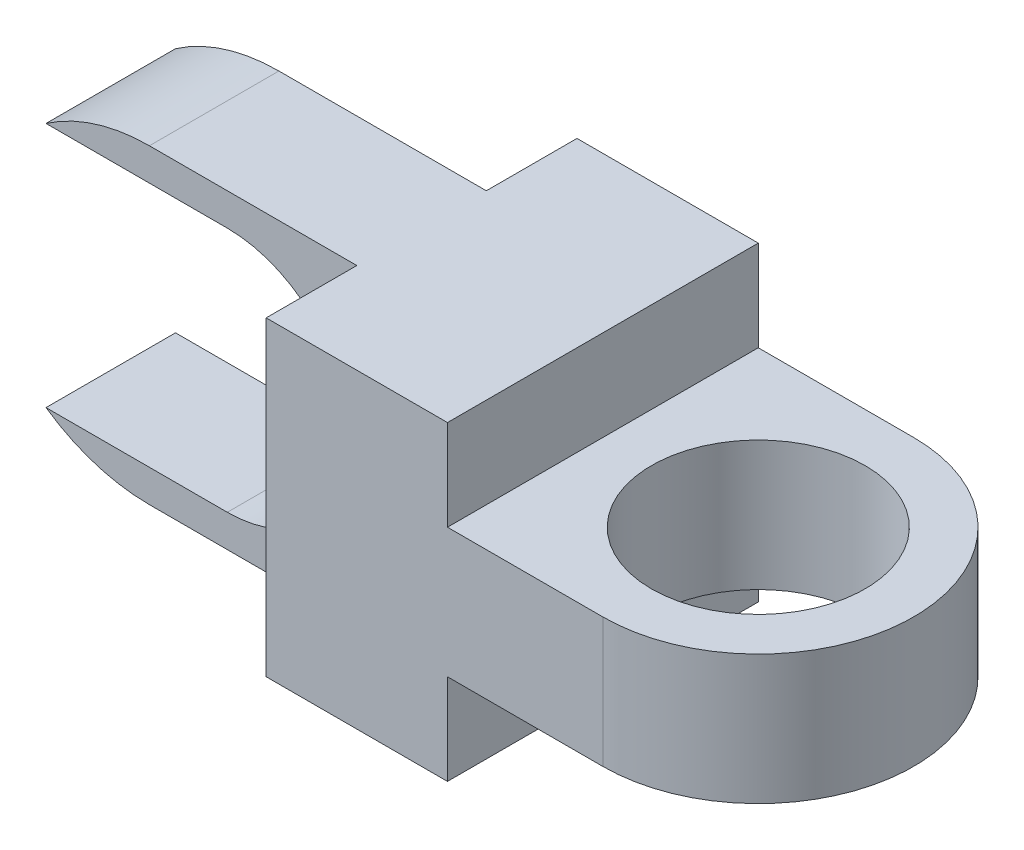
ISO-10303-21;
HEADER;
FILE_DESCRIPTION(('STEP AP214'),'2;1');
FILE_NAME('part.step','',(''),(''),'','','');
FILE_SCHEMA(('AUTOMOTIVE_DESIGN { 1 0 10303 214 1 1 1 1 }'));
ENDSEC;
DATA;
#1=APPLICATION_CONTEXT('core data for automotive mechanical design processes');
#2=APPLICATION_PROTOCOL_DEFINITION('international standard','automotive_design',2000,#1);
#3=PRODUCT_CONTEXT('',#1,'mechanical');
#4=PRODUCT('Part','Part','',(#3));
#5=PRODUCT_RELATED_PRODUCT_CATEGORY('part','',(#4));
#6=PRODUCT_DEFINITION_FORMATION('','',#4);
#7=PRODUCT_DEFINITION_CONTEXT('part definition',#1,'design');
#8=PRODUCT_DEFINITION('design','',#6,#7);
#9=PRODUCT_DEFINITION_SHAPE('','',#8);
#10=(LENGTH_UNIT() NAMED_UNIT(*) SI_UNIT(.MILLI.,.METRE.));
#11=(NAMED_UNIT(*) PLANE_ANGLE_UNIT() SI_UNIT($,.RADIAN.));
#12=(NAMED_UNIT(*) SI_UNIT($,.STERADIAN.) SOLID_ANGLE_UNIT());
#13=UNCERTAINTY_MEASURE_WITH_UNIT(LENGTH_MEASURE(1.E-05),#10,'distance_accuracy_value','');
#14=(GEOMETRIC_REPRESENTATION_CONTEXT(3) GLOBAL_UNCERTAINTY_ASSIGNED_CONTEXT((#13)) GLOBAL_UNIT_ASSIGNED_CONTEXT((#10,
#11,#12)) REPRESENTATION_CONTEXT('',''));
#15=CARTESIAN_POINT('',(0.,0.,0.));
#16=DIRECTION('',(0.,0.,1.));
#17=DIRECTION('',(1.,0.,0.));
#18=AXIS2_PLACEMENT_3D('',#15,#16,#17);
#19=CARTESIAN_POINT('',(0.,0.,24.));
#20=DIRECTION('',(1.,0.,0.));
#21=DIRECTION('',(0.,0.,-1.));
#22=AXIS2_PLACEMENT_3D('',#19,#20,#21);
#23=PLANE('',#22);
#24=DIRECTION('',(0.,1.,0.));
#25=VECTOR('',#24,1.);
#26=CARTESIAN_POINT('',(0.,0.,10.));
#27=LINE('',#26,#25);
#28=CARTESIAN_POINT('',(0.,-48.,10.));
#29=VERTEX_POINT('',#28);
#30=CARTESIAN_POINT('',(0.,0.,10.));
#31=VERTEX_POINT('',#30);
#32=EDGE_CURVE('E156',#29,#31,#27,.T.);
#33=ORIENTED_EDGE('',*,*,#32,.F.);
#34=DIRECTION('',(0.,0.,-1.));
#35=VECTOR('',#34,1.);
#36=CARTESIAN_POINT('',(0.,-48.,24.));
#37=LINE('',#36,#35);
#38=CARTESIAN_POINT('',(0.,-48.,24.));
#39=VERTEX_POINT('',#38);
#40=EDGE_CURVE('E11',#39,#29,#37,.T.);
#41=ORIENTED_EDGE('',*,*,#40,.F.);
#42=DIRECTION('',(0.,-1.,0.));
#43=VECTOR('',#42,1.);
#44=CARTESIAN_POINT('',(0.,0.,24.));
#45=LINE('',#44,#43);
#46=CARTESIAN_POINT('',(0.,0.,24.));
#47=VERTEX_POINT('',#46);
#48=EDGE_CURVE('E158',#47,#39,#45,.T.);
#49=ORIENTED_EDGE('',*,*,#48,.F.);
#50=DIRECTION('',(0.,0.,-1.));
#51=VECTOR('',#50,1.);
#52=CARTESIAN_POINT('',(0.,0.,24.));
#53=LINE('',#52,#51);
#54=EDGE_CURVE('E155',#47,#31,#53,.T.);
#55=ORIENTED_EDGE('',*,*,#54,.T.);
#56=EDGE_LOOP('',(#33,#41,#49,#55));
#57=FACE_BOUND('',#56,.T.);
#58=ADVANCED_FACE('F41',(#57),#23,.F.);
#59=CARTESIAN_POINT('',(28.,0.,24.));
#60=DIRECTION('',(-1.,0.,0.));
#61=DIRECTION('',(0.,-1.,0.));
#62=AXIS2_PLACEMENT_3D('',#59,#60,#61);
#63=PLANE('',#62);
#64=DIRECTION('',(0.,0.,1.));
#65=VECTOR('',#64,1.);
#66=CARTESIAN_POINT('',(28.,-14.,0.));
#67=LINE('',#66,#65);
#68=CARTESIAN_POINT('',(28.,-14.,-24.));
#69=VERTEX_POINT('',#68);
#70=CARTESIAN_POINT('',(28.,-14.,24.));
#71=VERTEX_POINT('',#70);
#72=EDGE_CURVE('E232',#69,#71,#67,.T.);
#73=ORIENTED_EDGE('',*,*,#72,.F.);
#74=DIRECTION('',(0.,1.,0.));
#75=VECTOR('',#74,1.);
#76=CARTESIAN_POINT('',(28.,0.,-24.));
#77=LINE('',#76,#75);
#78=CARTESIAN_POINT('',(28.,0.,-24.));
#79=VERTEX_POINT('',#78);
#80=EDGE_CURVE('E270',#69,#79,#77,.T.);
#81=ORIENTED_EDGE('',*,*,#80,.T.);
#82=DIRECTION('',(0.,0.,-1.));
#83=VECTOR('',#82,1.);
#84=CARTESIAN_POINT('',(28.,0.,24.));
#85=LINE('',#84,#83);
#86=CARTESIAN_POINT('',(28.,0.,24.));
#87=VERTEX_POINT('',#86);
#88=EDGE_CURVE('E161',#87,#79,#85,.T.);
#89=ORIENTED_EDGE('',*,*,#88,.F.);
#90=DIRECTION('',(0.,1.,0.));
#91=VECTOR('',#90,1.);
#92=CARTESIAN_POINT('',(28.,0.,24.));
#93=LINE('',#92,#91);
#94=EDGE_CURVE('E256',#71,#87,#93,.T.);
#95=ORIENTED_EDGE('',*,*,#94,.F.);
#96=EDGE_LOOP('',(#73,#81,#89,#95));
#97=FACE_BOUND('',#96,.T.);
#98=ADVANCED_FACE('F345',(#97),#63,.F.);
#99=CARTESIAN_POINT('',(0.,-48.,-10.));
#100=VERTEX_POINT('',#99);
#101=CARTESIAN_POINT('',(0.,-48.,-24.));
#102=VERTEX_POINT('',#101);
#103=EDGE_CURVE('E47',#100,#102,#37,.T.);
#104=ORIENTED_EDGE('',*,*,#103,.F.);
#105=DIRECTION('',(0.,1.,0.));
#106=VECTOR('',#105,1.);
#107=CARTESIAN_POINT('',(0.,0.,-10.));
#108=LINE('',#107,#106);
#109=CARTESIAN_POINT('',(0.,0.,-10.));
#110=VERTEX_POINT('',#109);
#111=EDGE_CURVE('E57',#100,#110,#108,.T.);
#112=ORIENTED_EDGE('',*,*,#111,.T.);
#113=CARTESIAN_POINT('',(0.,0.,-24.));
#114=VERTEX_POINT('',#113);
#115=EDGE_CURVE('E165',#110,#114,#53,.T.);
#116=ORIENTED_EDGE('',*,*,#115,.T.);
#117=DIRECTION('',(0.,-1.,0.));
#118=VECTOR('',#117,1.);
#119=CARTESIAN_POINT('',(0.,0.,-24.));
#120=LINE('',#119,#118);
#121=EDGE_CURVE('E251',#114,#102,#120,.T.);
#122=ORIENTED_EDGE('',*,*,#121,.T.);
#123=EDGE_LOOP('',(#104,#112,#116,#122));
#124=FACE_BOUND('',#123,.T.);
#125=ADVANCED_FACE('F43',(#124),#23,.F.);
#126=CARTESIAN_POINT('',(0.,-48.,24.));
#127=DIRECTION('',(0.,1.,0.));
#128=DIRECTION('',(0.,0.,1.));
#129=AXIS2_PLACEMENT_3D('',#126,#127,#128);
#130=PLANE('',#129);
#131=DIRECTION('',(1.,0.,0.));
#132=VECTOR('',#131,1.);
#133=CARTESIAN_POINT('',(0.,-48.,-24.));
#134=LINE('',#133,#132);
#135=CARTESIAN_POINT('',(28.,-48.,-24.));
#136=VERTEX_POINT('',#135);
#137=EDGE_CURVE('E264',#102,#136,#134,.T.);
#138=ORIENTED_EDGE('',*,*,#137,.T.);
#139=DIRECTION('',(0.,0.,-1.));
#140=VECTOR('',#139,1.);
#141=CARTESIAN_POINT('',(28.,-48.,24.));
#142=LINE('',#141,#140);
#143=CARTESIAN_POINT('',(28.,-48.,24.));
#144=VERTEX_POINT('',#143);
#145=EDGE_CURVE('E275',#144,#136,#142,.T.);
#146=ORIENTED_EDGE('',*,*,#145,.F.);
#147=DIRECTION('',(1.,0.,0.));
#148=VECTOR('',#147,1.);
#149=CARTESIAN_POINT('',(0.,-48.,24.));
#150=LINE('',#149,#148);
#151=EDGE_CURVE('E254',#39,#144,#150,.T.);
#152=ORIENTED_EDGE('',*,*,#151,.F.);
#153=ORIENTED_EDGE('',*,*,#40,.T.);
#154=DIRECTION('',(1.,0.,0.));
#155=VECTOR('',#154,1.);
#156=CARTESIAN_POINT('',(0.,-48.,10.));
#157=LINE('',#156,#155);
#158=CARTESIAN_POINT('',(-32.0312805773287,-48.,10.));
#159=VERTEX_POINT('',#158);
#160=EDGE_CURVE('E176',#159,#29,#157,.T.);
#161=ORIENTED_EDGE('',*,*,#160,.F.);
#162=DIRECTION('',(0.,0.,-1.));
#163=VECTOR('',#162,1.);
#164=CARTESIAN_POINT('',(-32.0312805773287,-48.,10.));
#165=LINE('',#164,#163);
#166=CARTESIAN_POINT('',(-32.0312805773287,-48.,-10.));
#167=VERTEX_POINT('',#166);
#168=EDGE_CURVE('E195',#159,#167,#165,.T.);
#169=ORIENTED_EDGE('',*,*,#168,.T.);
#170=DIRECTION('',(1.,0.,0.));
#171=VECTOR('',#170,1.);
#172=CARTESIAN_POINT('',(0.,-48.,-10.));
#173=LINE('',#172,#171);
#174=EDGE_CURVE('E180',#167,#100,#173,.T.);
#175=ORIENTED_EDGE('',*,*,#174,.T.);
#176=ORIENTED_EDGE('',*,*,#103,.T.);
#177=EDGE_LOOP('',(#138,#146,#152,#153,#161,#169,#175,#176));
#178=FACE_BOUND('',#177,.T.);
#179=ADVANCED_FACE('F278',(#178),#130,.F.);
#180=CARTESIAN_POINT('',(28.,-34.,-24.));
#181=VERTEX_POINT('',#180);
#182=EDGE_CURVE('E268',#136,#181,#77,.T.);
#183=ORIENTED_EDGE('',*,*,#182,.T.);
#184=DIRECTION('',(0.,0.,1.));
#185=VECTOR('',#184,1.);
#186=CARTESIAN_POINT('',(28.,-34.,0.));
#187=LINE('',#186,#185);
#188=CARTESIAN_POINT('',(28.,-34.,24.));
#189=VERTEX_POINT('',#188);
#190=EDGE_CURVE('E249',#181,#189,#187,.T.);
#191=ORIENTED_EDGE('',*,*,#190,.T.);
#192=EDGE_CURVE('E259',#144,#189,#93,.T.);
#193=ORIENTED_EDGE('',*,*,#192,.F.);
#194=ORIENTED_EDGE('',*,*,#145,.T.);
#195=EDGE_LOOP('',(#183,#191,#193,#194));
#196=FACE_BOUND('',#195,.T.);
#197=ADVANCED_FACE('F303',(#196),#63,.F.);
#198=CARTESIAN_POINT('',(0.,0.,24.));
#199=DIRECTION('',(0.,-1.,0.));
#200=DIRECTION('',(0.,0.,-1.));
#201=AXIS2_PLACEMENT_3D('',#198,#199,#200);
#202=PLANE('',#201);
#203=DIRECTION('',(-1.,0.,0.));
#204=VECTOR('',#203,1.);
#205=CARTESIAN_POINT('',(0.,0.,-24.));
#206=LINE('',#205,#204);
#207=EDGE_CURVE('E258',#79,#114,#206,.T.);
#208=ORIENTED_EDGE('',*,*,#207,.T.);
#209=ORIENTED_EDGE('',*,*,#115,.F.);
#210=DIRECTION('',(-1.,0.,0.));
#211=VECTOR('',#210,1.);
#212=CARTESIAN_POINT('',(0.,0.,-10.));
#213=LINE('',#212,#211);
#214=CARTESIAN_POINT('',(-32.0312805773287,0.,-10.));
#215=VERTEX_POINT('',#214);
#216=EDGE_CURVE('E192',#110,#215,#213,.T.);
#217=ORIENTED_EDGE('',*,*,#216,.T.);
#218=DIRECTION('',(0.,0.,-1.));
#219=VECTOR('',#218,1.);
#220=CARTESIAN_POINT('',(-32.0312805773287,0.,10.));
#221=LINE('',#220,#219);
#222=CARTESIAN_POINT('',(-32.0312805773287,0.,10.));
#223=VERTEX_POINT('',#222);
#224=EDGE_CURVE('E166',#223,#215,#221,.T.);
#225=ORIENTED_EDGE('',*,*,#224,.F.);
#226=DIRECTION('',(-1.,0.,0.));
#227=VECTOR('',#226,1.);
#228=CARTESIAN_POINT('',(0.,0.,10.));
#229=LINE('',#228,#227);
#230=EDGE_CURVE('E164',#31,#223,#229,.T.);
#231=ORIENTED_EDGE('',*,*,#230,.F.);
#232=ORIENTED_EDGE('',*,*,#54,.F.);
#233=DIRECTION('',(-1.,0.,0.));
#234=VECTOR('',#233,1.);
#235=CARTESIAN_POINT('',(0.,0.,24.));
#236=LINE('',#235,#234);
#237=EDGE_CURVE('E265',#87,#47,#236,.T.);
#238=ORIENTED_EDGE('',*,*,#237,.F.);
#239=ORIENTED_EDGE('',*,*,#88,.T.);
#240=EDGE_LOOP('',(#208,#209,#217,#225,#231,#232,#238,#239));
#241=FACE_BOUND('',#240,.T.);
#242=ADVANCED_FACE('F170',(#241),#202,.F.);
#243=CARTESIAN_POINT('',(0.,0.,24.));
#244=DIRECTION('',(0.,0.,1.));
#245=DIRECTION('',(1.,0.,0.));
#246=AXIS2_PLACEMENT_3D('',#243,#244,#245);
#247=PLANE('',#246);
#248=ORIENTED_EDGE('',*,*,#48,.T.);
#249=ORIENTED_EDGE('',*,*,#151,.T.);
#250=ORIENTED_EDGE('',*,*,#192,.T.);
#251=DIRECTION('',(1.,0.,0.));
#252=VECTOR('',#251,1.);
#253=CARTESIAN_POINT('',(0.,-34.,24.));
#254=LINE('',#253,#252);
#255=CARTESIAN_POINT('',(52.,-34.,24.));
#256=VERTEX_POINT('',#255);
#257=EDGE_CURVE('E231',#189,#256,#254,.T.);
#258=ORIENTED_EDGE('',*,*,#257,.T.);
#259=DIRECTION('',(0.,-1.,0.));
#260=VECTOR('',#259,1.);
#261=CARTESIAN_POINT('',(52.,-14.,24.));
#262=LINE('',#261,#260);
#263=CARTESIAN_POINT('',(52.,-14.,24.));
#264=VERTEX_POINT('',#263);
#265=EDGE_CURVE('E238',#264,#256,#262,.T.);
#266=ORIENTED_EDGE('',*,*,#265,.F.);
#267=DIRECTION('',(1.,0.,0.));
#268=VECTOR('',#267,1.);
#269=CARTESIAN_POINT('',(0.,-14.,24.));
#270=LINE('',#269,#268);
#271=EDGE_CURVE('E236',#71,#264,#270,.T.);
#272=ORIENTED_EDGE('',*,*,#271,.F.);
#273=ORIENTED_EDGE('',*,*,#94,.T.);
#274=ORIENTED_EDGE('',*,*,#237,.T.);
#275=EDGE_LOOP('',(#248,#249,#250,#258,#266,#272,#273,#274));
#276=FACE_BOUND('',#275,.T.);
#277=ADVANCED_FACE('F308',(#276),#247,.T.);
#278=CARTESIAN_POINT('',(0.,0.,-24.));
#279=DIRECTION('',(0.,0.,1.));
#280=DIRECTION('',(1.,0.,0.));
#281=AXIS2_PLACEMENT_3D('',#278,#279,#280);
#282=PLANE('',#281);
#283=ORIENTED_EDGE('',*,*,#121,.F.);
#284=ORIENTED_EDGE('',*,*,#207,.F.);
#285=ORIENTED_EDGE('',*,*,#80,.F.);
#286=DIRECTION('',(-1.,0.,0.));
#287=VECTOR('',#286,1.);
#288=CARTESIAN_POINT('',(0.,-14.,-24.));
#289=LINE('',#288,#287);
#290=CARTESIAN_POINT('',(52.,-14.,-24.));
#291=VERTEX_POINT('',#290);
#292=EDGE_CURVE('E234',#291,#69,#289,.T.);
#293=ORIENTED_EDGE('',*,*,#292,.F.);
#294=DIRECTION('',(0.,-1.,0.));
#295=VECTOR('',#294,1.);
#296=CARTESIAN_POINT('',(52.,-14.,-24.));
#297=LINE('',#296,#295);
#298=CARTESIAN_POINT('',(52.,-34.,-24.));
#299=VERTEX_POINT('',#298);
#300=EDGE_CURVE('E253',#291,#299,#297,.T.);
#301=ORIENTED_EDGE('',*,*,#300,.T.);
#302=DIRECTION('',(-1.,0.,0.));
#303=VECTOR('',#302,1.);
#304=CARTESIAN_POINT('',(0.,-34.,-24.));
#305=LINE('',#304,#303);
#306=EDGE_CURVE('E242',#299,#181,#305,.T.);
#307=ORIENTED_EDGE('',*,*,#306,.T.);
#308=ORIENTED_EDGE('',*,*,#182,.F.);
#309=ORIENTED_EDGE('',*,*,#137,.F.);
#310=EDGE_LOOP('',(#283,#284,#285,#293,#301,#307,#308,#309));
#311=FACE_BOUND('',#310,.T.);
#312=ADVANCED_FACE('F283',(#311),#282,.F.);
#313=CARTESIAN_POINT('',(52.,-14.,0.));
#314=DIRECTION('',(0.,-1.,0.));
#315=DIRECTION('',(0.,0.,-1.));
#316=AXIS2_PLACEMENT_3D('',#313,#314,#315);
#317=CYLINDRICAL_SURFACE('',#316,24.);
#318=CARTESIAN_POINT('',(52.,-34.,0.));
#319=DIRECTION('',(0.,1.,0.));
#320=DIRECTION('',(0.,0.,1.));
#321=AXIS2_PLACEMENT_3D('',#318,#319,#320);
#322=CIRCLE('',#321,24.);
#323=EDGE_CURVE('E223',#299,#256,#322,.F.);
#324=ORIENTED_EDGE('',*,*,#323,.F.);
#325=ORIENTED_EDGE('',*,*,#300,.F.);
#326=CARTESIAN_POINT('',(52.,-14.,0.));
#327=DIRECTION('',(0.,1.,0.));
#328=DIRECTION('',(0.,0.,1.));
#329=AXIS2_PLACEMENT_3D('',#326,#327,#328);
#330=CIRCLE('',#329,24.);
#331=EDGE_CURVE('E227',#291,#264,#330,.F.);
#332=ORIENTED_EDGE('',*,*,#331,.T.);
#333=ORIENTED_EDGE('',*,*,#265,.T.);
#334=EDGE_LOOP('',(#324,#325,#332,#333));
#335=FACE_BOUND('',#334,.T.);
#336=ADVANCED_FACE('F297',(#335),#317,.T.);
#337=CARTESIAN_POINT('',(0.,-14.,0.));
#338=DIRECTION('',(0.,1.,0.));
#339=DIRECTION('',(0.,0.,1.));
#340=AXIS2_PLACEMENT_3D('',#337,#338,#339);
#341=PLANE('',#340);
#342=CARTESIAN_POINT('',(52.,-14.,0.));
#343=DIRECTION('',(0.,1.,0.));
#344=DIRECTION('',(0.,0.,1.));
#345=AXIS2_PLACEMENT_3D('',#342,#343,#344);
#346=CIRCLE('',#345,16.5);
#347=CARTESIAN_POINT('',(52.,-14.,16.5));
#348=VERTEX_POINT('',#347);
#349=EDGE_CURVE('E222',#348,#348,#346,.T.);
#350=ORIENTED_EDGE('',*,*,#349,.F.);
#351=EDGE_LOOP('',(#350));
#352=FACE_BOUND('',#351,.T.);
#353=ORIENTED_EDGE('',*,*,#331,.F.);
#354=ORIENTED_EDGE('',*,*,#292,.T.);
#355=ORIENTED_EDGE('',*,*,#72,.T.);
#356=ORIENTED_EDGE('',*,*,#271,.T.);
#357=EDGE_LOOP('',(#353,#354,#355,#356));
#358=FACE_BOUND('',#357,.T.);
#359=ADVANCED_FACE('F291',(#352,#358),#341,.T.);
#360=CARTESIAN_POINT('',(0.,-34.,0.));
#361=DIRECTION('',(0.,1.,0.));
#362=DIRECTION('',(0.,0.,1.));
#363=AXIS2_PLACEMENT_3D('',#360,#361,#362);
#364=PLANE('',#363);
#365=CARTESIAN_POINT('',(52.,-34.,0.));
#366=DIRECTION('',(0.,1.,0.));
#367=DIRECTION('',(0.,0.,1.));
#368=AXIS2_PLACEMENT_3D('',#365,#366,#367);
#369=CIRCLE('',#368,16.5);
#370=CARTESIAN_POINT('',(52.,-34.,16.5));
#371=VERTEX_POINT('',#370);
#372=EDGE_CURVE('E225',#371,#371,#369,.T.);
#373=ORIENTED_EDGE('',*,*,#372,.T.);
#374=EDGE_LOOP('',(#373));
#375=FACE_BOUND('',#374,.T.);
#376=ORIENTED_EDGE('',*,*,#323,.T.);
#377=ORIENTED_EDGE('',*,*,#257,.F.);
#378=ORIENTED_EDGE('',*,*,#190,.F.);
#379=ORIENTED_EDGE('',*,*,#306,.F.);
#380=EDGE_LOOP('',(#376,#377,#378,#379));
#381=FACE_BOUND('',#380,.T.);
#382=ADVANCED_FACE('F301',(#375,#381),#364,.F.);
#383=CARTESIAN_POINT('',(52.,-34.,0.));
#384=DIRECTION('',(0.,1.,0.));
#385=DIRECTION('',(0.,0.,1.));
#386=AXIS2_PLACEMENT_3D('',#383,#384,#385);
#387=CYLINDRICAL_SURFACE('',#386,16.5);
#388=ORIENTED_EDGE('',*,*,#372,.F.);
#389=EDGE_LOOP('',(#388));
#390=FACE_BOUND('',#389,.T.);
#391=ORIENTED_EDGE('',*,*,#349,.T.);
#392=EDGE_LOOP('',(#391));
#393=FACE_BOUND('',#392,.T.);
#394=ADVANCED_FACE('F370',(#390,#393),#387,.F.);
#395=CARTESIAN_POINT('',(-32.0312805773287,-28.,10.));
#396=DIRECTION('',(0.,0.,-1.));
#397=DIRECTION('',(-1.,0.,0.));
#398=AXIS2_PLACEMENT_3D('',#395,#396,#397);
#399=CYLINDRICAL_SURFACE('',#398,28.);
#400=CARTESIAN_POINT('',(-32.0312805773287,-28.,-10.));
#401=DIRECTION('',(0.,0.,1.));
#402=DIRECTION('',(-1.,0.,0.));
#403=AXIS2_PLACEMENT_3D('',#400,#401,#402);
#404=CIRCLE('',#403,28.);
#405=CARTESIAN_POINT('',(-48.,-5.,-10.));
#406=VERTEX_POINT('',#405);
#407=EDGE_CURVE('E197',#215,#406,#404,.T.);
#408=ORIENTED_EDGE('',*,*,#407,.T.);
#409=DIRECTION('',(0.,0.,-1.));
#410=VECTOR('',#409,1.);
#411=CARTESIAN_POINT('',(-48.,-5.,10.));
#412=LINE('',#411,#410);
#413=CARTESIAN_POINT('',(-48.,-5.,10.));
#414=VERTEX_POINT('',#413);
#415=EDGE_CURVE('E220',#414,#406,#412,.T.);
#416=ORIENTED_EDGE('',*,*,#415,.F.);
#417=CARTESIAN_POINT('',(-32.0312805773287,-28.,10.));
#418=DIRECTION('',(0.,0.,1.));
#419=DIRECTION('',(-1.,0.,0.));
#420=AXIS2_PLACEMENT_3D('',#417,#418,#419);
#421=CIRCLE('',#420,28.);
#422=EDGE_CURVE('E175',#223,#414,#421,.T.);
#423=ORIENTED_EDGE('',*,*,#422,.F.);
#424=ORIENTED_EDGE('',*,*,#224,.T.);
#425=EDGE_LOOP('',(#408,#416,#423,#424));
#426=FACE_BOUND('',#425,.T.);
#427=ADVANCED_FACE('F320',(#426),#399,.T.);
#428=CARTESIAN_POINT('',(-20.,-5.,10.));
#429=DIRECTION('',(0.,1.,0.));
#430=DIRECTION('',(0.,0.,1.));
#431=AXIS2_PLACEMENT_3D('',#428,#429,#430);
#432=PLANE('',#431);
#433=DIRECTION('',(1.,0.,0.));
#434=VECTOR('',#433,1.);
#435=CARTESIAN_POINT('',(-20.,-5.,-10.));
#436=LINE('',#435,#434);
#437=CARTESIAN_POINT('',(-20.,-5.,-10.));
#438=VERTEX_POINT('',#437);
#439=EDGE_CURVE('E200',#406,#438,#436,.T.);
#440=ORIENTED_EDGE('',*,*,#439,.T.);
#441=DIRECTION('',(0.,0.,-1.));
#442=VECTOR('',#441,1.);
#443=CARTESIAN_POINT('',(-20.,-5.,10.));
#444=LINE('',#443,#442);
#445=CARTESIAN_POINT('',(-20.,-5.,10.));
#446=VERTEX_POINT('',#445);
#447=EDGE_CURVE('E212',#446,#438,#444,.T.);
#448=ORIENTED_EDGE('',*,*,#447,.F.);
#449=DIRECTION('',(1.,0.,0.));
#450=VECTOR('',#449,1.);
#451=CARTESIAN_POINT('',(-20.,-5.,10.));
#452=LINE('',#451,#450);
#453=EDGE_CURVE('E184',#414,#446,#452,.T.);
#454=ORIENTED_EDGE('',*,*,#453,.F.);
#455=ORIENTED_EDGE('',*,*,#415,.T.);
#456=EDGE_LOOP('',(#440,#448,#454,#455));
#457=FACE_BOUND('',#456,.T.);
#458=ADVANCED_FACE('F322',(#457),#432,.F.);
#459=CARTESIAN_POINT('',(-20.,-24.,10.));
#460=DIRECTION('',(0.,0.,-1.));
#461=DIRECTION('',(-1.,0.,0.));
#462=AXIS2_PLACEMENT_3D('',#459,#460,#461);
#463=CYLINDRICAL_SURFACE('',#462,19.);
#464=CARTESIAN_POINT('',(-20.,-24.,-10.));
#465=DIRECTION('',(0.,0.,-1.));
#466=DIRECTION('',(1.,0.,0.));
#467=AXIS2_PLACEMENT_3D('',#464,#465,#466);
#468=CIRCLE('',#467,19.);
#469=CARTESIAN_POINT('',(-20.,-43.,-10.));
#470=VERTEX_POINT('',#469);
#471=EDGE_CURVE('E203',#438,#470,#468,.T.);
#472=ORIENTED_EDGE('',*,*,#471,.T.);
#473=DIRECTION('',(0.,0.,-1.));
#474=VECTOR('',#473,1.);
#475=CARTESIAN_POINT('',(-20.,-43.,10.));
#476=LINE('',#475,#474);
#477=CARTESIAN_POINT('',(-20.,-43.,10.));
#478=VERTEX_POINT('',#477);
#479=EDGE_CURVE('E211',#478,#470,#476,.T.);
#480=ORIENTED_EDGE('',*,*,#479,.F.);
#481=CARTESIAN_POINT('',(-20.,-24.,10.));
#482=DIRECTION('',(0.,0.,-1.));
#483=DIRECTION('',(1.,0.,0.));
#484=AXIS2_PLACEMENT_3D('',#481,#482,#483);
#485=CIRCLE('',#484,19.);
#486=EDGE_CURVE('E186',#446,#478,#485,.T.);
#487=ORIENTED_EDGE('',*,*,#486,.F.);
#488=ORIENTED_EDGE('',*,*,#447,.T.);
#489=EDGE_LOOP('',(#472,#480,#487,#488));
#490=FACE_BOUND('',#489,.T.);
#491=ADVANCED_FACE('F330',(#490),#463,.F.);
#492=CARTESIAN_POINT('',(-20.,-43.,10.));
#493=DIRECTION('',(0.,-1.,0.));
#494=DIRECTION('',(0.,0.,-1.));
#495=AXIS2_PLACEMENT_3D('',#492,#493,#494);
#496=PLANE('',#495);
#497=DIRECTION('',(-1.,0.,0.));
#498=VECTOR('',#497,1.);
#499=CARTESIAN_POINT('',(-20.,-43.,-10.));
#500=LINE('',#499,#498);
#501=CARTESIAN_POINT('',(-48.,-43.,-10.));
#502=VERTEX_POINT('',#501);
#503=EDGE_CURVE('E201',#470,#502,#500,.T.);
#504=ORIENTED_EDGE('',*,*,#503,.T.);
#505=DIRECTION('',(0.,0.,-1.));
#506=VECTOR('',#505,1.);
#507=CARTESIAN_POINT('',(-48.,-43.,10.));
#508=LINE('',#507,#506);
#509=CARTESIAN_POINT('',(-48.,-43.,10.));
#510=VERTEX_POINT('',#509);
#511=EDGE_CURVE('E208',#510,#502,#508,.T.);
#512=ORIENTED_EDGE('',*,*,#511,.F.);
#513=DIRECTION('',(-1.,0.,0.));
#514=VECTOR('',#513,1.);
#515=CARTESIAN_POINT('',(-20.,-43.,10.));
#516=LINE('',#515,#514);
#517=EDGE_CURVE('E187',#478,#510,#516,.T.);
#518=ORIENTED_EDGE('',*,*,#517,.F.);
#519=ORIENTED_EDGE('',*,*,#479,.T.);
#520=EDGE_LOOP('',(#504,#512,#518,#519));
#521=FACE_BOUND('',#520,.T.);
#522=ADVANCED_FACE('F332',(#521),#496,.F.);
#523=CARTESIAN_POINT('',(-32.0312805773287,-20.,10.));
#524=DIRECTION('',(0.,0.,-1.));
#525=DIRECTION('',(-1.,0.,0.));
#526=AXIS2_PLACEMENT_3D('',#523,#524,#525);
#527=CYLINDRICAL_SURFACE('',#526,28.);
#528=CARTESIAN_POINT('',(-32.0312805773287,-20.,-10.));
#529=DIRECTION('',(0.,0.,1.));
#530=DIRECTION('',(1.,0.,0.));
#531=AXIS2_PLACEMENT_3D('',#528,#529,#530);
#532=CIRCLE('',#531,28.);
#533=EDGE_CURVE('E177',#502,#167,#532,.T.);
#534=ORIENTED_EDGE('',*,*,#533,.T.);
#535=ORIENTED_EDGE('',*,*,#168,.F.);
#536=CARTESIAN_POINT('',(-32.0312805773287,-20.,10.));
#537=DIRECTION('',(0.,0.,1.));
#538=DIRECTION('',(1.,0.,0.));
#539=AXIS2_PLACEMENT_3D('',#536,#537,#538);
#540=CIRCLE('',#539,28.);
#541=EDGE_CURVE('E189',#510,#159,#540,.T.);
#542=ORIENTED_EDGE('',*,*,#541,.F.);
#543=ORIENTED_EDGE('',*,*,#511,.T.);
#544=EDGE_LOOP('',(#534,#535,#542,#543));
#545=FACE_BOUND('',#544,.T.);
#546=ADVANCED_FACE('F335',(#545),#527,.T.);
#547=CARTESIAN_POINT('',(-32.0312805773287,-20.,10.));
#548=DIRECTION('',(0.,0.,1.));
#549=DIRECTION('',(1.,0.,0.));
#550=AXIS2_PLACEMENT_3D('',#547,#548,#549);
#551=PLANE('',#550);
#552=ORIENTED_EDGE('',*,*,#32,.T.);
#553=ORIENTED_EDGE('',*,*,#230,.T.);
#554=ORIENTED_EDGE('',*,*,#422,.T.);
#555=ORIENTED_EDGE('',*,*,#453,.T.);
#556=ORIENTED_EDGE('',*,*,#486,.T.);
#557=ORIENTED_EDGE('',*,*,#517,.T.);
#558=ORIENTED_EDGE('',*,*,#541,.T.);
#559=ORIENTED_EDGE('',*,*,#160,.T.);
#560=EDGE_LOOP('',(#552,#553,#554,#555,#556,#557,#558,#559));
#561=FACE_BOUND('',#560,.T.);
#562=ADVANCED_FACE('F174',(#561),#551,.T.);
#563=CARTESIAN_POINT('',(-32.0312805773287,-20.,-10.));
#564=DIRECTION('',(0.,0.,1.));
#565=DIRECTION('',(1.,0.,0.));
#566=AXIS2_PLACEMENT_3D('',#563,#564,#565);
#567=PLANE('',#566);
#568=ORIENTED_EDGE('',*,*,#111,.F.);
#569=ORIENTED_EDGE('',*,*,#174,.F.);
#570=ORIENTED_EDGE('',*,*,#533,.F.);
#571=ORIENTED_EDGE('',*,*,#503,.F.);
#572=ORIENTED_EDGE('',*,*,#471,.F.);
#573=ORIENTED_EDGE('',*,*,#439,.F.);
#574=ORIENTED_EDGE('',*,*,#407,.F.);
#575=ORIENTED_EDGE('',*,*,#216,.F.);
#576=EDGE_LOOP('',(#568,#569,#570,#571,#572,#573,#574,#575));
#577=FACE_BOUND('',#576,.T.);
#578=ADVANCED_FACE('F315',(#577),#567,.F.);
#579=CLOSED_SHELL('',(#58,#98,#125,#179,#197,#242,#277,#312,#336,#359,#382,#394,#427,#458,#491,
#522,#546,#562,#578));
#580=MANIFOLD_SOLID_BREP('B2',#579);
#581=ADVANCED_BREP_SHAPE_REPRESENTATION('',(#18,#580),#14);
#582=SHAPE_DEFINITION_REPRESENTATION(#9,#581);
ENDSEC;
END-ISO-10303-21;
